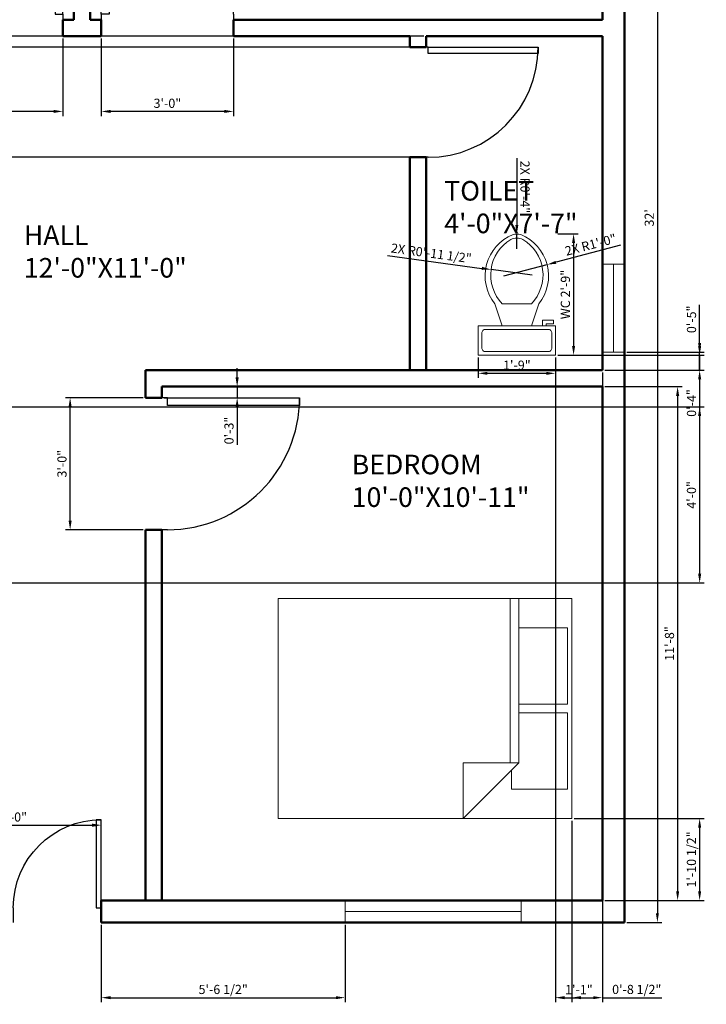
# Model space of a CAD drawing. Units: inches. Extents: x 158445 to 158806, y 254100 to 254533.
# Tile 2 of 3: x 158619 to 158806, y 254100 to 254369. Entities that reach past the tile are written whole.
import ezdxf

# ---------------------------------------------------------------- set-up
doc = ezdxf.new("R2010")
doc.units = ezdxf.units.IN
for name, color, linetype, lineweight in [('A-ANNO-DIMS', 2, 'Continuous', 18), ('A-AREA-IDEN', 7, 'Continuous', 25), ('A-DOOR', 3, 'Continuous', 25), ('A-FLOR-FIXT', 9, 'Continuous', 18), ('A-FURN', 8, 'Continuous', 18), ('A-GLAZ', 4, 'Continuous', 18), ('A-WALL', 7, 'Continuous', 50)]:
    doc.layers.add(name, color=color, linetype=linetype, lineweight=lineweight)
doc.styles.get("Standard").update_dxf_attribs({"font": 'arial.ttf'})
doc.dimstyles.new('ISO-25', dxfattribs={"dimtxt": 2.5, "dimasz": 2.5, "dimexe": 1.25, "dimexo": 0.625, "dimtad": 1, "dimlunit": 4, "dimtxsty": 'Standard', "dimcen": 2.5, "dimadec": 0, "dimazin": 0, "dimtfac": 1, "dimtmove": 0, "dimatfit": 3, "dimfxl": 1, "dimarcsym": 0})

# ---------------------------------------------------------------- blocks, each defined once
blk = doc.blocks.new('*U2')
for p, q in [((0, 0), (0, -5)), ((30, 0), (30, -5))]:
    blk.add_line(p, q)
blk.add_lwpolyline([(0, 0), (0, 30), (1.75, 30), (1.75, 0)], close=True)
blk.add_arc((0, 0), 30, 0, 90)
blk = doc.blocks.new('Bed - Queen')
for p, q in [((0, -80.00003), (0, 0)), ((0, 0), (59.99999, 0)), ((59.99999, 0), (59.99999, -80.00003)), ((7.99999, -1.2), (28.79998, -1.2)), ((7.99999, -14.4), (7.99999, -1.2)), ((28.79998, -1.2), (28.79998, -14.4)), ((31.19999, -1.2), (51.99999, -1.2)), ((31.19999, -14.4), (31.19999, -1.2)), ((51.99999, -1.2), (51.99999, -16.4)), ((0, -14.4), (44.8, -14.4)), ((59.99999, -29.6), (44.8, -14.4)), ((44.8, -14.4), (44.8, -29.6)), ((44.8, -16.8), (0, -16.8)), ((51.99999, -16.4), (46.79936, -16.4)), ((44.8, -29.6), (59.99999, -29.6)), ((59.99999, -80.00003), (0, -80.00003))]:
    blk.add_line(p, q)
blk = doc.blocks.new('Toilet - top')
for p, q in [((9.5, -6), (9.5, -2)), ((-8, -8.5), (-8, -8)), ((-7, -8), (-7, -9.5)), ((-4, -8), (-6, -14)), ((4, -8), (6, -14)), ((-10, -8.5), (-8, -8.5)), ((-10, -9.5), (-10, -8.5)), ((-7, -9.5), (-10, -9.5)), ((4, -14), (-4, -14))]:
    blk.add_line(p, q)
blk.add_lwpolyline([(10.5, -8), (10.5, 0), (-10.5, 0), (-10.5, -8)], close=True)
for points in [[(-9.5, -2), (-9.5, -6)], [(8.5, -1), (-8.5, -1)], [(-8.5, -7), (8.5, -7)]]:
    blk.add_lwpolyline(points)
for centre, radius, start, end in [((-8.62, -1.88), 0.884, 81.8699, 188.1301), ((8.62, -1.88), 0.884, 351.8699, 98.1301), ((-8.62, -6.12), 0.884, 171.8699, 278.1301), ((8.62, -6.12), 0.884, 261.8699, 8.1301), ((3.52, -21.58), 12.17, 141.4691, 247.9714), ((4.2, -21.82), 11.33, 136.3677, 238.9468), ((-3.52, -21.58), 12.17, 292.0284, 38.5307), ((-4.2, -21.82), 11.33, 301.053, 43.6321), ((0, -27.88), 4, 245.7318, 294.2682), ((0, -29), 4, 254.8605, 285.1395)]:
    blk.add_arc(centre, radius, start, end)
blk = doc.blocks.new('*D7')
at = {"layer": 'A-ANNO-DIMS', "color": 0, "lineweight": -2, "transparency": 16777216}
for p, q in [((158784.01, 254506.72), (158793.62, 254506.72)), ((158792.37, 254504.22), (158792.37, 254125.22)), ((158784.01, 254122.72), (158793.62, 254122.72))]:
    blk.add_line(p, q, dxfattribs=at)
at = {"layer": 'A-ANNO-DIMS', "color": 0, "transparency": 16777216}
for points in [[(158791.95, 254504.22), (158792.78, 254504.22), (158792.37, 254506.72)], [(158791.95, 254125.22), (158792.78, 254125.22), (158792.37, 254122.72)]]:
    blk.add_solid(points, dxfattribs=at)
at = {"layer": 'Defpoints', "color": 0, "transparency": 16777216}
for p in [(158783.38, 254506.72), (158783.38, 254122.72), (158792.37, 254122.72)]:
    blk.add_point(p, dxfattribs=at)
at = {"layer": 'A-ANNO-DIMS', "color": 0, "transparency": 16777216, "insert": (158790.47, 254314.72), "char_height": 2.5, "attachment_point": 5, "rotation": 90}
blk.add_mtext("32'", dxfattribs=at)
blk = doc.blocks.new('WIN-48IN')
for p, q in [((0, 6), (0, 0)), ((48, 6), (48, 0)), ((0, 3), (48, 3))]:
    blk.add_line(p, q)
blk = doc.blocks.new('WIN-24IN')
for p, q in [((0, 24), (6, 24)), ((3, 0), (3, 24)), ((0, 0), (6, 0))]:
    blk.add_line(p, q)
blk = doc.blocks.new('*D16')
at = {"layer": 'A-ANNO-DIMS', "color": 0, "lineweight": -2, "transparency": 16777216}
for p, q in [((158765.2, 254310.35), (158770.79, 254310.35)), ((158769.54, 254307.85), (158769.54, 254279.8)), ((158765.2, 254277.3), (158770.79, 254277.3))]:
    blk.add_line(p, q, dxfattribs=at)
at = {"layer": 'A-ANNO-DIMS', "color": 0, "transparency": 16777216}
for points in [[(158769.12, 254307.85), (158769.95, 254307.85), (158769.54, 254310.35)], [(158769.12, 254279.8), (158769.95, 254279.8), (158769.54, 254277.3)]]:
    blk.add_solid(points, dxfattribs=at)
at = {"layer": 'Defpoints', "color": 0, "transparency": 16777216}
for p in [(158764.58, 254310.35), (158764.58, 254277.3), (158769.54, 254277.3)]:
    blk.add_point(p, dxfattribs=at)
at = {"layer": 'A-ANNO-DIMS', "color": 0, "transparency": 16777216, "insert": (158767.62, 254293.83), "char_height": 2.5, "attachment_point": 5, "rotation": 90}
blk.add_mtext('WC 2\'-9"', dxfattribs=at)
blk = doc.blocks.new('*D17')
at = {"layer": 'A-ANNO-DIMS', "color": 0, "lineweight": -2, "transparency": 16777216}
for p, q in [((158743.58, 254276.68), (158743.58, 254271.1)), ((158764.58, 254276.68), (158764.58, 254271.1)), ((158762.08, 254272.35), (158746.08, 254272.35))]:
    blk.add_line(p, q, dxfattribs=at)
at = {"layer": 'A-ANNO-DIMS', "color": 0, "transparency": 16777216}
for points in [[(158746.08, 254272.76), (158746.08, 254271.93), (158743.58, 254272.35)], [(158762.08, 254272.76), (158762.08, 254271.93), (158764.58, 254272.35)]]:
    blk.add_solid(points, dxfattribs=at)
at = {"layer": 'Defpoints', "color": 0, "transparency": 16777216}
for p in [(158743.58, 254277.3), (158764.58, 254277.3), (158743.58, 254272.35)]:
    blk.add_point(p, dxfattribs=at)
at = {"layer": 'A-ANNO-DIMS', "color": 0, "transparency": 16777216, "insert": (158754.08, 254274.25), "char_height": 2.5, "attachment_point": 5}
blk.add_mtext('1\'-9"', dxfattribs=at)
blk = doc.blocks.new('*D22')
at = {"layer": 'A-ANNO-DIMS', "color": 0, "lineweight": -2, "transparency": 16777216}
for p, q in [((158803.88, 254280.62), (158803.88, 254291.02)), ((158784.01, 254278.12), (158805.13, 254278.12)), ((158803.88, 254273.22), (158803.88, 254278.12)), ((158778.01, 254273.22), (158805.13, 254273.22)), ((158803.88, 254270.72), (158803.88, 254268.22))]:
    blk.add_line(p, q, dxfattribs=at)
at = {"layer": 'A-ANNO-DIMS', "color": 0, "transparency": 16777216}
for points in [[(158803.46, 254280.62), (158804.3, 254280.62), (158803.88, 254278.12)], [(158803.46, 254270.72), (158804.3, 254270.72), (158803.88, 254273.22)]]:
    blk.add_solid(points, dxfattribs=at)
at = {"layer": 'Defpoints', "color": 0, "transparency": 16777216}
for p in [(158783.38, 254278.12), (158803.88, 254278.12), (158777.38, 254273.22)]:
    blk.add_point(p, dxfattribs=at)
at = {"layer": 'A-ANNO-DIMS', "color": 0, "transparency": 16777216, "insert": (158801.98, 254287.07), "char_height": 2.5, "attachment_point": 5, "rotation": 90}
blk.add_mtext('0\'-5"', dxfattribs=at)
blk = doc.blocks.new('*D25')
at = {"layer": 'A-ANNO-DIMS', "color": 0, "lineweight": -2, "transparency": 16777216}
for p, q in [((158592.88, 254129.35), (158592.88, 254150.47)), ((158595.38, 254149.22), (158638.38, 254149.22)), ((158640.88, 254129.35), (158640.88, 254150.47))]:
    blk.add_line(p, q, dxfattribs=at)
at = {"layer": 'A-ANNO-DIMS', "color": 0, "transparency": 16777216}
for points in [[(158595.38, 254149.64), (158595.38, 254148.8), (158592.88, 254149.22)], [(158638.38, 254149.64), (158638.38, 254148.8), (158640.88, 254149.22)]]:
    blk.add_solid(points, dxfattribs=at)
at = {"layer": 'Defpoints', "color": 0, "transparency": 16777216}
for p in [(158640.88, 254149.22), (158592.88, 254128.72), (158640.88, 254128.72)]:
    blk.add_point(p, dxfattribs=at)
at = {"layer": 'A-ANNO-DIMS', "color": 0, "transparency": 16777216, "insert": (158616.88, 254151.12), "char_height": 2.5, "attachment_point": 5}
blk.add_mtext('4\'-0"', dxfattribs=at)
blk = doc.blocks.new('*D26')
at = {"layer": 'A-ANNO-DIMS', "color": 0, "lineweight": -2, "transparency": 16777216}
for p, q in [((158640.88, 254122.1), (158640.88, 254100.97)), ((158707.27, 254122.1), (158707.27, 254100.97)), ((158643.38, 254102.22), (158704.77, 254102.22))]:
    blk.add_line(p, q, dxfattribs=at)
at = {"layer": 'A-ANNO-DIMS', "color": 0, "transparency": 16777216}
for points in [[(158643.38, 254102.64), (158643.38, 254101.8), (158640.88, 254102.22)], [(158704.77, 254102.64), (158704.77, 254101.8), (158707.27, 254102.22)]]:
    blk.add_solid(points, dxfattribs=at)
at = {"layer": 'Defpoints', "color": 0, "transparency": 16777216}
for p in [(158640.88, 254122.72), (158707.27, 254122.72), (158707.27, 254102.22)]:
    blk.add_point(p, dxfattribs=at)
at = {"layer": 'A-ANNO-DIMS', "color": 0, "transparency": 16777216, "insert": (158674.08, 254104.14), "char_height": 2.5, "attachment_point": 5}
blk.add_mtext('5\'-6 1/2"', dxfattribs=at)
blk = doc.blocks.new('*D28')
at = {"layer": 'A-ANNO-DIMS', "color": 0, "lineweight": -2, "transparency": 16777216}
for p, q in [((158778.01, 254268.72), (158799.13, 254268.72)), ((158797.88, 254266.22), (158797.88, 254131.22)), ((158778.01, 254128.72), (158799.13, 254128.72))]:
    blk.add_line(p, q, dxfattribs=at)
at = {"layer": 'A-ANNO-DIMS', "color": 0, "transparency": 16777216}
for points in [[(158797.46, 254266.22), (158798.3, 254266.22), (158797.88, 254268.72)], [(158797.46, 254131.22), (158798.3, 254131.22), (158797.88, 254128.72)]]:
    blk.add_solid(points, dxfattribs=at)
at = {"layer": 'Defpoints', "color": 0, "transparency": 16777216}
for p in [(158777.38, 254268.72), (158777.38, 254128.72), (158797.88, 254128.72)]:
    blk.add_point(p, dxfattribs=at)
at = {"layer": 'A-ANNO-DIMS', "color": 0, "transparency": 16777216, "insert": (158795.98, 254198.72), "char_height": 2.5, "attachment_point": 5, "rotation": 90}
blk.add_mtext('11\'-8"', dxfattribs=at)
blk = doc.blocks.new('*D29')
at = {"layer": 'A-ANNO-DIMS', "color": 0, "lineweight": -2, "transparency": 16777216}
for p, q in [((158728.76, 254361.22), (158449.63, 254361.22)), ((158450.88, 254333.72), (158450.88, 254358.72)), ((158728.76, 254331.22), (158449.63, 254331.22))]:
    blk.add_line(p, q, dxfattribs=at)
at = {"layer": 'A-ANNO-DIMS', "color": 0, "transparency": 16777216}
for points in [[(158450.46, 254358.72), (158451.3, 254358.72), (158450.88, 254361.22)], [(158450.46, 254333.72), (158451.3, 254333.72), (158450.88, 254331.22)]]:
    blk.add_solid(points, dxfattribs=at)
at = {"layer": 'Defpoints', "color": 0, "transparency": 16777216}
for p in [(158450.88, 254361.22), (158729.38, 254361.22), (158729.38, 254331.22)]:
    blk.add_point(p, dxfattribs=at)
at = {"layer": 'A-ANNO-DIMS', "color": 0, "transparency": 16777216, "insert": (158448.98, 254346.22), "char_height": 2.5, "attachment_point": 5, "rotation": 90}
blk.add_mtext('2\'-6"', dxfattribs=at)
blk = doc.blocks.new('*D34')
at = {"layer": 'A-ANNO-DIMS', "color": 0, "lineweight": -2, "transparency": 16777216}
for p, q in [((158554.01, 254263.22), (158805.13, 254263.22)), ((158803.88, 254260.72), (158803.88, 254217.72)), ((158554.01, 254215.22), (158805.13, 254215.22))]:
    blk.add_line(p, q, dxfattribs=at)
at = {"layer": 'A-ANNO-DIMS', "color": 0, "transparency": 16777216}
for points in [[(158803.46, 254260.72), (158804.3, 254260.72), (158803.88, 254263.22)], [(158803.46, 254217.72), (158804.3, 254217.72), (158803.88, 254215.22)]]:
    blk.add_solid(points, dxfattribs=at)
at = {"layer": 'Defpoints', "color": 0, "transparency": 16777216}
for p in [(158553.38, 254263.22), (158553.38, 254215.22), (158803.88, 254215.22)]:
    blk.add_point(p, dxfattribs=at)
at = {"layer": 'A-ANNO-DIMS', "color": 0, "transparency": 16777216, "insert": (158801.98, 254239.22), "char_height": 2.5, "attachment_point": 5, "rotation": 90}
blk.add_mtext('4\'-0"', dxfattribs=at)
blk = doc.blocks.new('*D38')
at = {"layer": 'A-ANNO-DIMS', "color": 0, "lineweight": -2, "transparency": 16777216}
for p, q in [((158764.58, 254276.68), (158764.58, 254100.97)), ((158777.38, 254272.6), (158777.38, 254100.97)), ((158767.08, 254102.22), (158774.88, 254102.22))]:
    blk.add_line(p, q, dxfattribs=at)
at = {"layer": 'A-ANNO-DIMS', "color": 0, "transparency": 16777216}
for points in [[(158767.08, 254102.64), (158767.08, 254101.8), (158764.58, 254102.22)], [(158774.88, 254102.64), (158774.88, 254101.8), (158777.38, 254102.22)]]:
    blk.add_solid(points, dxfattribs=at)
at = {"layer": 'Defpoints', "color": 0, "transparency": 16777216}
for p in [(158764.58, 254277.3), (158777.38, 254273.22), (158777.38, 254102.22)]:
    blk.add_point(p, dxfattribs=at)
at = {"layer": 'A-ANNO-DIMS', "color": 0, "transparency": 16777216, "insert": (158770.98, 254104.1), "char_height": 2.5, "attachment_point": 5}
blk.add_mtext('1\'-1"', dxfattribs=at)
blk = doc.blocks.new('*D39')
at = {"layer": 'A-ANNO-DIMS', "color": 0, "lineweight": -2, "transparency": 16777216}
for p, q in [((158803.88, 254279.8), (158803.88, 254282.3)), ((158765.2, 254277.3), (158805.13, 254277.3)), ((158803.88, 254277.3), (158803.88, 254273.22)), ((158778.01, 254273.22), (158805.13, 254273.22)), ((158803.88, 254270.72), (158803.88, 254260.33))]:
    blk.add_line(p, q, dxfattribs=at)
at = {"layer": 'A-ANNO-DIMS', "color": 0, "transparency": 16777216}
for points in [[(158803.46, 254279.8), (158804.3, 254279.8), (158803.88, 254277.3)], [(158803.46, 254270.72), (158804.3, 254270.72), (158803.88, 254273.22)]]:
    blk.add_solid(points, dxfattribs=at)
at = {"layer": 'Defpoints', "color": 0, "transparency": 16777216}
for p in [(158764.58, 254277.3), (158777.38, 254273.22), (158803.88, 254273.22)]:
    blk.add_point(p, dxfattribs=at)
at = {"layer": 'A-ANNO-DIMS', "color": 0, "transparency": 16777216, "insert": (158801.98, 254264.27), "char_height": 2.5, "attachment_point": 5, "rotation": 90}
blk.add_mtext('0\'-4"', dxfattribs=at)
blk = doc.blocks.new('*D40')
at = {"layer": 'A-ANNO-DIMS', "color": 0, "lineweight": -2, "transparency": 16777216}
for p, q in [((158594.38, 254363.6), (158594.38, 254342.47)), ((158630.38, 254363.6), (158630.38, 254342.47)), ((158627.88, 254343.72), (158596.88, 254343.72))]:
    blk.add_line(p, q, dxfattribs=at)
at = {"layer": 'A-ANNO-DIMS', "color": 0, "transparency": 16777216}
for points in [[(158596.88, 254344.14), (158596.88, 254343.3), (158594.38, 254343.72)], [(158627.88, 254344.14), (158627.88, 254343.3), (158630.38, 254343.72)]]:
    blk.add_solid(points, dxfattribs=at)
at = {"layer": 'Defpoints', "color": 0, "transparency": 16777216}
for p in [(158594.38, 254364.22), (158630.38, 254364.22), (158594.38, 254343.72)]:
    blk.add_point(p, dxfattribs=at)
at = {"layer": 'A-ANNO-DIMS', "color": 0, "transparency": 16777216, "insert": (158612.38, 254345.62), "char_height": 2.5, "attachment_point": 5}
blk.add_mtext('3\'-0"', dxfattribs=at)
blk = doc.blocks.new('*D41')
at = {"layer": 'A-ANNO-DIMS', "color": 0, "lineweight": -2, "transparency": 16777216}
for p, q in [((158640.88, 254363.6), (158640.88, 254342.47)), ((158676.88, 254363.6), (158676.88, 254342.47)), ((158674.38, 254343.72), (158643.38, 254343.72))]:
    blk.add_line(p, q, dxfattribs=at)
at = {"layer": 'A-ANNO-DIMS', "color": 0, "transparency": 16777216}
for points in [[(158643.38, 254344.14), (158643.38, 254343.3), (158640.88, 254343.72)], [(158674.38, 254344.14), (158674.38, 254343.3), (158676.88, 254343.72)]]:
    blk.add_solid(points, dxfattribs=at)
at = {"layer": 'Defpoints', "color": 0, "transparency": 16777216}
for p in [(158640.88, 254364.22), (158676.88, 254364.22), (158640.88, 254343.72)]:
    blk.add_point(p, dxfattribs=at)
at = {"layer": 'A-ANNO-DIMS', "color": 0, "transparency": 16777216, "insert": (158658.88, 254345.62), "char_height": 2.5, "attachment_point": 5}
blk.add_mtext('3\'-0"', dxfattribs=at)
blk = doc.blocks.new('*D43')
at = {"layer": 'A-ANNO-DIMS', "color": 0, "lineweight": -2, "transparency": 16777216}
for p, q in [((158652.26, 254265.72), (158631.13, 254265.72)), ((158632.38, 254232.22), (158632.38, 254263.22)), ((158652.26, 254229.72), (158631.13, 254229.72))]:
    blk.add_line(p, q, dxfattribs=at)
at = {"layer": 'A-ANNO-DIMS', "color": 0, "transparency": 16777216}
for points in [[(158631.96, 254263.22), (158632.8, 254263.22), (158632.38, 254265.72)], [(158631.96, 254232.22), (158632.8, 254232.22), (158632.38, 254229.72)]]:
    blk.add_solid(points, dxfattribs=at)
at = {"layer": 'Defpoints', "color": 0, "transparency": 16777216}
for p in [(158632.38, 254265.72), (158652.88, 254265.72), (158652.88, 254229.72)]:
    blk.add_point(p, dxfattribs=at)
at = {"layer": 'A-ANNO-DIMS', "color": 0, "transparency": 16777216, "insert": (158630.48, 254247.72), "char_height": 2.5, "attachment_point": 5, "rotation": 90}
blk.add_mtext('3\'-0"', dxfattribs=at)
blk = doc.blocks.new('*D49')
at = {"layer": 'A-ANNO-DIMS', "color": 0, "lineweight": -2, "transparency": 16777216}
for p, q in [((158769.68, 254151.03), (158805.13, 254151.03)), ((158803.88, 254148.53), (158803.88, 254131.22)), ((158778.01, 254128.72), (158805.13, 254128.72))]:
    blk.add_line(p, q, dxfattribs=at)
at = {"layer": 'A-ANNO-DIMS', "color": 0, "transparency": 16777216}
for points in [[(158803.46, 254148.53), (158804.3, 254148.53), (158803.88, 254151.03)], [(158803.46, 254131.22), (158804.3, 254131.22), (158803.88, 254128.72)]]:
    blk.add_solid(points, dxfattribs=at)
at = {"layer": 'Defpoints', "color": 0, "transparency": 16777216}
for p in [(158769.06, 254151.03), (158777.38, 254128.72), (158803.88, 254128.72)]:
    blk.add_point(p, dxfattribs=at)
at = {"layer": 'A-ANNO-DIMS', "color": 0, "transparency": 16777216, "insert": (158801.96, 254139.88), "char_height": 2.5, "attachment_point": 5, "rotation": 90}
blk.add_mtext('1\'-10 1/2"', dxfattribs=at)
blk = doc.blocks.new('*D50')
at = {"layer": 'A-ANNO-DIMS', "color": 0, "lineweight": -2, "transparency": 16777216}
for p, q in [((158769.06, 254150.41), (158769.06, 254100.97)), ((158777.38, 254128.1), (158777.38, 254100.97)), ((158771.56, 254102.22), (158774.88, 254102.22)), ((158777.38, 254102.22), (158793.6, 254102.22))]:
    blk.add_line(p, q, dxfattribs=at)
at = {"layer": 'A-ANNO-DIMS', "color": 0, "transparency": 16777216}
for points in [[(158771.56, 254102.64), (158771.56, 254101.8), (158769.06, 254102.22)], [(158774.88, 254102.64), (158774.88, 254101.8), (158777.38, 254102.22)]]:
    blk.add_solid(points, dxfattribs=at)
at = {"layer": 'Defpoints', "color": 0, "transparency": 16777216}
for p in [(158769.06, 254151.03), (158777.38, 254128.72), (158777.38, 254102.22)]:
    blk.add_point(p, dxfattribs=at)
at = {"layer": 'A-ANNO-DIMS', "color": 0, "transparency": 16777216, "insert": (158786.74, 254104.14), "char_height": 2.5, "attachment_point": 5}
blk.add_mtext('0\'-8 1/2"', dxfattribs=at)
blk = doc.blocks.new('*D52')
at = {"layer": 'A-ANNO-DIMS', "color": 0, "lineweight": -2, "transparency": 16777216}
for p, q in [((158677.88, 254271.22), (158677.88, 254273.72)), ((158658.01, 254268.72), (158679.13, 254268.72)), ((158677.88, 254268.72), (158677.88, 254265.72)), ((158658.01, 254265.72), (158679.13, 254265.72)), ((158677.88, 254263.22), (158677.88, 254252.83))]:
    blk.add_line(p, q, dxfattribs=at)
at = {"layer": 'A-ANNO-DIMS', "color": 0, "transparency": 16777216}
for points in [[(158677.46, 254271.22), (158678.3, 254271.22), (158677.88, 254268.72)], [(158677.46, 254263.22), (158678.3, 254263.22), (158677.88, 254265.72)]]:
    blk.add_solid(points, dxfattribs=at)
at = {"layer": 'Defpoints', "color": 0, "transparency": 16777216}
for p in [(158657.38, 254268.72), (158657.38, 254265.72), (158677.88, 254265.72)]:
    blk.add_point(p, dxfattribs=at)
at = {"layer": 'A-ANNO-DIMS', "color": 0, "transparency": 16777216, "insert": (158675.98, 254256.77), "char_height": 2.5, "attachment_point": 5, "rotation": 90}
blk.add_mtext('0\'-3"', dxfattribs=at)
blk = doc.blocks.new('*D53')
at = {"layer": 'A-ANNO-DIMS', "color": 0, "lineweight": -2, "transparency": 16777216}
for p, q in [((158450.88, 254366.72), (158450.88, 254377.12)), ((158728.76, 254364.22), (158449.63, 254364.22)), ((158450.88, 254361.22), (158450.88, 254364.22)), ((158728.76, 254361.22), (158449.63, 254361.22)), ((158450.88, 254358.72), (158450.88, 254356.22))]:
    blk.add_line(p, q, dxfattribs=at)
at = {"layer": 'A-ANNO-DIMS', "color": 0, "transparency": 16777216}
for points in [[(158450.46, 254366.72), (158451.3, 254366.72), (158450.88, 254364.22)], [(158450.46, 254358.72), (158451.3, 254358.72), (158450.88, 254361.22)]]:
    blk.add_solid(points, dxfattribs=at)
at = {"layer": 'Defpoints', "color": 0, "transparency": 16777216}
for p in [(158450.88, 254364.22), (158729.38, 254364.22), (158729.38, 254361.22)]:
    blk.add_point(p, dxfattribs=at)
at = {"layer": 'A-ANNO-DIMS', "color": 0, "transparency": 16777216, "insert": (158448.98, 254373.17), "char_height": 2.5, "attachment_point": 5, "rotation": 90}
blk.add_mtext('0\'-3"', dxfattribs=at)
blk = doc.blocks.new('*D54')
at = {"layer": 'A-ANNO-DIMS', "color": 0, "lineweight": -2, "transparency": 16777216}
for p, q in [((158782.35, 254307.24), (158764.75, 254302.61)), ((158750.56, 254298.88), (158762.33, 254301.98))]:
    blk.add_line(p, q, dxfattribs=at)
at = {"layer": 'A-ANNO-DIMS', "color": 0, "transparency": 16777216}
blk.add_solid([(158764.64, 254303.01), (158764.85, 254302.21), (158762.33, 254301.98)], dxfattribs=at)
at = {"layer": 'Defpoints', "color": 0, "transparency": 16777216}
for p in [(158762.33, 254301.98), (158750.56, 254298.88)]:
    blk.add_point(p, dxfattribs=at)
at = {"layer": 'A-ANNO-DIMS', "color": 0, "transparency": 16777216, "insert": (158774.27, 254307.08), "char_height": 2.5, "attachment_point": 5, "rotation": 14.7194}
blk.add_mtext('2X R1\'-0"', dxfattribs=at)
blk = doc.blocks.new('*D55')
at = {"layer": 'A-ANNO-DIMS', "color": 0, "lineweight": -2, "transparency": 16777216}
for p, q in [((158718.83, 254304.42), (158744.57, 254300.96)), ((158758.28, 254299.12), (158747.05, 254300.63))]:
    blk.add_line(p, q, dxfattribs=at)
at = {"layer": 'A-ANNO-DIMS', "color": 0, "transparency": 16777216}
blk.add_solid([(158744.63, 254301.38), (158744.52, 254300.55), (158747.05, 254300.63)], dxfattribs=at)
at = {"layer": 'Defpoints', "color": 0, "transparency": 16777216}
for p in [(158747.05, 254300.63), (158758.28, 254299.12)]:
    blk.add_point(p, dxfattribs=at)
at = {"layer": 'A-ANNO-DIMS', "color": 0, "transparency": 16777216, "insert": (158730.72, 254304.76), "char_height": 2.5, "attachment_point": 5, "rotation": 352.3408}
blk.add_mtext('2X R0\'-11 1/2"', dxfattribs=at)
blk = doc.blocks.new('*D56')
at = {"layer": 'A-ANNO-DIMS', "color": 0, "lineweight": -2, "transparency": 16777216}
for p, q in [((158754.08, 254331.01), (158754.08, 254312.8)), ((158754.08, 254306.3), (158754.08, 254310.3))]:
    blk.add_line(p, q, dxfattribs=at)
at = {"layer": 'A-ANNO-DIMS', "color": 0, "transparency": 16777216}
blk.add_solid([(158754.49, 254312.8), (158753.66, 254312.8), (158754.08, 254310.3)], dxfattribs=at)
at = {"layer": 'Defpoints', "color": 0, "transparency": 16777216}
for p in [(158754.08, 254310.3), (158754.08, 254306.3)]:
    blk.add_point(p, dxfattribs=at)
at = {"layer": 'A-ANNO-DIMS', "color": 0, "transparency": 16777216, "insert": (158755.98, 254323.15), "char_height": 2.5, "attachment_point": 5, "rotation": 270.0041}
blk.add_mtext('2X R0\'-4"', dxfattribs=at)

msp = doc.modelspace()

# ---------------------------------------------------------------- linework, layer by layer
at = {"layer": 'A-WALL'}
for p, q in [((158783.381, 254122.721), (158783.381, 254506.721)), ((158633.381, 254500.721), (158633.381, 254368.721)), ((158637.881, 254500.721), (158637.881, 254368.721)), ((158777.381, 254368.721), (158777.381, 254500.721)), ((158633.381, 254368.721), (158630.381, 254368.721)), ((158633.381, 254368.721), (158630.381, 254368.721)), ((158630.381, 254368.721), (158630.381, 254364.221)), ((158637.881, 254368.721), (158640.881, 254368.721)), ((158640.881, 254368.721), (158637.881, 254368.721)), ((158640.881, 254368.721), (158640.881, 254364.221)), ((158777.381, 254368.721), (158676.881, 254368.721)), ((158676.881, 254364.221), (158676.881, 254368.721)), ((158640.881, 254364.221), (158630.381, 254364.221)), ((158724.881, 254364.221), (158676.881, 254364.221)), ((158724.881, 254364.221), (158724.881, 254361.221)), ((158724.881, 254361.221), (158724.881, 254364.221)), ((158777.381, 254364.221), (158729.381, 254364.221)), ((158729.381, 254361.221), (158729.381, 254364.221)), ((158777.381, 254273.221), (158777.381, 254364.221)), ((158724.881, 254361.221), (158729.381, 254361.221)), ((158724.881, 254273.221), (158724.881, 254331.221)), ((158729.381, 254331.221), (158724.881, 254331.221)), ((158729.381, 254273.221), (158729.381, 254331.221)), ((158777.381, 254273.221), (158652.881, 254273.221)), ((158652.881, 254265.721), (158652.881, 254273.221)), ((158777.381, 254268.721), (158657.381, 254268.721)), ((158657.381, 254268.721), (158657.381, 254265.721)), ((158657.381, 254265.721), (158657.381, 254268.721)), ((158777.381, 254128.721), (158777.381, 254268.721)), ((158657.381, 254265.721), (158652.881, 254265.721)), ((158652.881, 254128.721), (158652.881, 254229.721)), ((158652.881, 254229.721), (158657.381, 254229.721)), ((158657.381, 254128.721), (158657.381, 254229.721)), ((158652.881, 254128.721), (158640.881, 254128.721)), ((158640.881, 254128.721), (158640.881, 254122.721)), ((158640.881, 254128.721), (158777.381, 254128.721)), ((158640.881, 254122.721), (158783.381, 254122.721))]:
    msp.add_line(p, q, dxfattribs=at)

# ---------------------------------------------------------------- block references
at = {"layer": 'A-DOOR'}
for p, xscale, yscale, zscale in [((158630.381, 254370.221), -1.199999999999999, 1.199999999999999, 1.199999999999999), ((158640.881, 254370.221), 1.199999999999999, 1.199999999999999, 1.199999999999999), ((158640.881, 254126.721), -0.8, 0.8, 0.8)]:
    msp.add_blockref('*U2', p, dxfattribs=dict(at, xscale=xscale, yscale=yscale, zscale=zscale))
at = {"layer": 'A-DOOR', "rotation": 270}
msp.add_blockref('*U2', (158729.881, 254361.221), dxfattribs=at)
at = {"layer": 'A-DOOR', "xscale": 1.199999999999999, "yscale": 1.199999999999999, "zscale": 1.199999999999999, "rotation": 270}
msp.add_blockref('*U2', (158658.881, 254265.721), dxfattribs=at)
at = {"layer": 'A-FLOR-FIXT', "rotation": 180}
msp.add_blockref('Toilet - top', (158754.078, 254277.303), dxfattribs=at)
at = {"layer": 'A-FURN', "rotation": 270}
msp.add_blockref('Bed - Queen', (158769.06, 254211.033), dxfattribs=at)
at = {"layer": 'A-GLAZ'}
for name, p in [('WIN-24IN', (158777.381, 254278.121)), ('WIN-48IN', (158707.272, 254122.721))]:
    msp.add_blockref(name, p, dxfattribs=at)

# ---------------------------------------------------------------- texts
at = {"layer": 'A-AREA-IDEN', "char_height": 5.335, "attachment_point": 1}
for s, insert in [('TOILET\\P4\'-0"X7\'-7"', (158734.292, 254324.767)), ('HALL\\P12\'-0"X11\'-0"', (158619.762, 254312.669)), ('BEDROOM\\P10\'-0"X10\'-11"', (158709.087, 254250.177))]:
    msp.add_mtext_dynamic_manual_height_columns(s, width=5.37287, gutter_width=26.675, heights=[0], dxfattribs=dict(at, insert=insert))

# ---------------------------------------------------------------- dimensions: what is measured, and where the dimension line sits
at = {"layer": 'A-ANNO-DIMS'}
for base, p1, p2, angle, override, picture, middle in [((158792.368, 254122.721), (158783.381, 254506.721), (158783.381, 254122.721), 90, {"dimclrd": 0, "dimclre": 0, "dimclrt": 0}, '*D7', (158790.465, 254314.721)), ((158450.881, 254364.221), (158729.381, 254361.221), (158729.381, 254364.221), 90, {"dimdec": 1, "dimlfac": 1, "dimrnd": 0, "dimzin": 1, "dimdsep": 46, "dimlunit": 4, "dimfrac": 2}, '*D53', (158448.979, 254373.169)), ((158594.381, 254343.721), (158630.381, 254364.221), (158594.381, 254364.221), 180, {"dimdec": 1, "dimlfac": 1, "dimrnd": 0, "dimzin": 1, "dimdsep": 46, "dimlunit": 4, "dimfrac": 2}, '*D40', (158612.381, 254345.623)), ((158640.881, 254343.721), (158676.881, 254364.221), (158640.881, 254364.221), 180, {"dimdec": 1, "dimlfac": 1, "dimrnd": 0, "dimzin": 1, "dimdsep": 46, "dimlunit": 4, "dimfrac": 2}, '*D41', (158658.881, 254345.623)), ((158450.881, 254361.221), (158729.381, 254331.221), (158729.381, 254361.221), 90, {"dimdec": 1, "dimlfac": 1, "dimrnd": 0, "dimzin": 1, "dimdsep": 46, "dimlunit": 4, "dimfrac": 2}, '*D29', (158448.98, 254346.221)), ((158803.881, 254278.121), (158777.381, 254273.221), (158783.381, 254278.121), 90, {"dimdec": 1, "dimlfac": 1, "dimrnd": 0, "dimzin": 1, "dimdsep": 46, "dimlunit": 4, "dimfrac": 2}, '*D22', (158801.98, 254287.069)), ((158803.881, 254273.221), (158764.578, 254277.303), (158777.381, 254273.221), 90, {"dimdec": 1, "dimlfac": 1, "dimrnd": 0, "dimzin": 1, "dimdsep": 46, "dimlunit": 4, "dimfrac": 2}, '*D39', (158801.98, 254264.273)), ((158743.578, 254272.346), (158764.578, 254277.303), (158743.578, 254277.303), 180, {"dimdec": 1, "dimlfac": 1, "dimrnd": 0, "dimzin": 1, "dimdsep": 46, "dimlunit": 4, "dimfrac": 2}, '*D17', (158754.078, 254274.247)), ((158677.881, 254265.721), (158657.381, 254268.721), (158657.381, 254265.721), 270, {"dimdec": 1, "dimlfac": 1, "dimrnd": 0, "dimzin": 1, "dimdsep": 46, "dimlunit": 4, "dimfrac": 2}, '*D52', (158675.979, 254256.773)), ((158797.881, 254128.721), (158777.381, 254268.721), (158777.381, 254128.721), 270, {"dimdec": 1, "dimlfac": 1, "dimrnd": 0, "dimzin": 1, "dimdsep": 46, "dimlunit": 4, "dimfrac": 2}, '*D28', (158795.98, 254198.721)), ((158632.381, 254265.721), (158652.881, 254229.721), (158652.881, 254265.721), 90, {"dimdec": 1, "dimlfac": 1, "dimrnd": 0, "dimzin": 1, "dimdsep": 46, "dimlunit": 4, "dimfrac": 2}, '*D43', (158630.479, 254247.721)), ((158803.881, 254215.221), (158553.381, 254263.221), (158553.381, 254215.221), 90, {"dimdec": 1, "dimlfac": 1, "dimrnd": 0, "dimzin": 1, "dimdsep": 46, "dimlunit": 4, "dimfrac": 2}, '*D34', (158801.98, 254239.221)), ((158803.881, 254128.721), (158769.06, 254151.033), (158777.381, 254128.721), 90, {"dimdec": 1, "dimlfac": 1, "dimrnd": 0, "dimzin": 1, "dimdsep": 46, "dimlunit": 4, "dimfrac": 2}, '*D49', (158801.964, 254139.877))]:
    dim = msp.add_linear_dim(base=base, p1=p1, p2=p2, angle=angle, dimstyle='ISO-25', override=override, dxfattribs=at)
    dim.commit()
    dim.dimension.update_dxf_attribs({"geometry": picture, "text_midpoint": middle})
for center, mpoint, picture, middle in [((158754.078, 254306.303), (158754.078, 254310.303), '*D56', (158755.979, 254323.154)), ((158758.278, 254299.12), (158747.05, 254300.63), '*D55', (158730.72, 254304.761)), ((158750.559, 254298.883), (158762.328, 254301.975), '*D54', (158774.275, 254307.079))]:
    dim = msp.add_radius_dim(center=center, mpoint=mpoint, text='2X <>', dimstyle='ISO-25', override={"dimdec": 1, "dimlfac": 1, "dimrnd": 0, "dimzin": 1, "dimdsep": 46, "dimlunit": 4, "dimfrac": 2}, dxfattribs=at)
    dim.commit()
    dim.dimension.update_dxf_attribs({"geometry": picture, "text_midpoint": middle})
dim = msp.add_linear_dim(base=(158769.535, 254277.303), p1=(158764.578, 254310.349), p2=(158764.578, 254277.303), angle=270, text='WC <>', dimstyle='ISO-25', override={"dimdec": 1, "dimlfac": 1, "dimrnd": 0, "dimzin": 1, "dimdsep": 46, "dimlunit": 4, "dimfrac": 2}, dxfattribs=at)
dim.commit()
dim.dimension.update_dxf_attribs({"geometry": '*D16', "text_midpoint": (158767.618, 254293.826)})
for base, p1, p2, picture, middle in [((158777.381, 254102.221), (158764.578, 254277.303), (158777.381, 254273.221), '*D38', (158770.98, 254104.101)), ((158640.881, 254149.221), (158592.881, 254128.721), (158640.881, 254128.721), '*D25', (158616.881, 254151.122)), ((158777.381, 254102.221), (158769.06, 254151.033), (158777.381, 254128.721), '*D50', (158786.742, 254104.139)), ((158707.272, 254102.221), (158640.881, 254122.721), (158707.272, 254122.721), '*D26', (158674.077, 254104.139))]:
    dim = msp.add_linear_dim(base=base, p1=p1, p2=p2, dimstyle='ISO-25', override={"dimdec": 1, "dimlfac": 1, "dimrnd": 0, "dimzin": 1, "dimdsep": 46, "dimlunit": 4, "dimfrac": 2}, dxfattribs=at)
    dim.commit()
    dim.dimension.update_dxf_attribs({"geometry": picture, "text_midpoint": middle})

doc.saveas('drawing.dxf')
